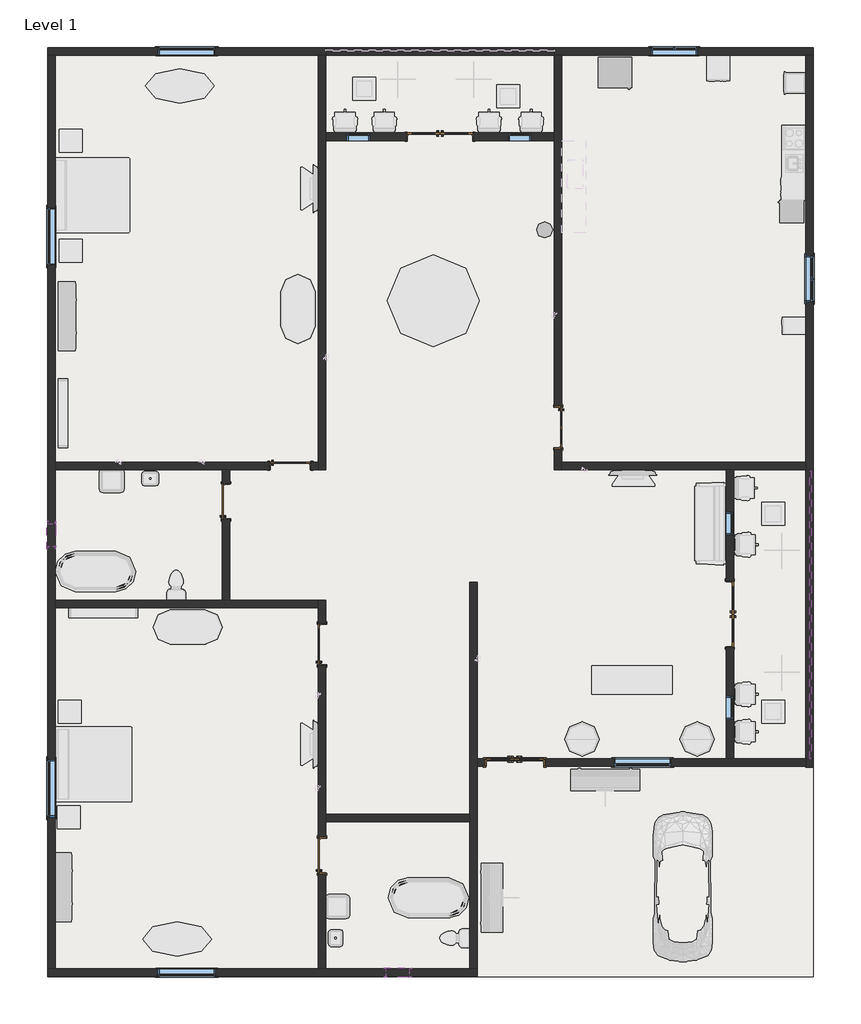
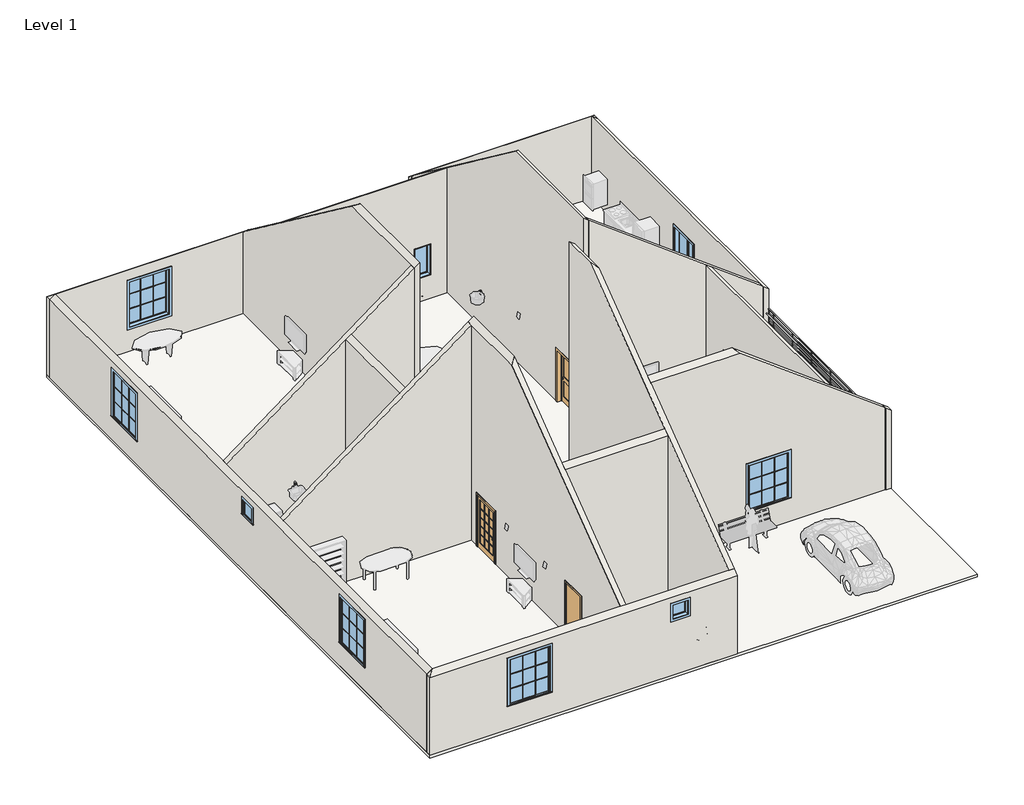
# One storey, part 1 of 2: 20 walls, 13 windows, 8 doors, 1 railing, 1 slab.
"""IFC4 building model written with IfcOpenShell, lengths in millimetres."""

from ifc_helpers import new_model, si_unit, point, frame, frame_2d, origin, origin_with_axes, place, context, project, spatial, polyline, circle_curve, trimmed, segment, composite_curve, outline, extrude, faceted_brep, transform, mapped, element, save
from components import door_b03bd389, door_146fce4d, door_63baf7d0, door_797b0c7a, door_f3911013, window_cc15f82e, window_0862ab64, window_9110666e, window_80bd9af0, window_e41d21a6

model = new_model("IFC4")

# Units and contexts
model_context = context("Model", 3, world=origin())
ifc_project = project(units=[si_unit("LENGTHUNIT", "METRE", prefix="MILLI")], contexts=[model_context])

# Site, building, storey
site = spatial("IfcSite", under=ifc_project)
building = spatial("IfcBuilding", under=site)
storey = spatial("IfcBuildingStorey", under=building, Name="Level 1", Elevation=0.0)

# Doors
placement = place(None, origin())
door_shape = door_b03bd389(model_context)
element("IfcDoor", 1, ObjectType="Door-Exterior-Double-Full Glass-Wood_Clad : 60\" x 80\"", at=placement, inside=storey, context=model_context, shape_type="MappedRepresentation", body=[
    mapped(door_shape, transform((-2295.8295712, -8019.3204109, 0.0), x_axis=(1.0, 0.0, 0.0), y_axis=(0.0, 1.0, 0.0), z_axis=(0.0, 0.0, 1.0))),
])
door_2_shape = door_146fce4d(model_context)
element("IfcDoor", 2, ObjectType="Door-Interior-Double-Full Glass-Wood : 68\" x 80\"", at=placement, inside=storey, context=model_context, shape_type="MappedRepresentation", body=[
    mapped(door_2_shape, transform((-4277.0295712, 8541.4795891, 0.0), x_axis=(1.0, 0.0, 0.0), y_axis=(0.0, 1.0, 0.0), z_axis=(0.0, 0.0, 1.0))),
])
element("IfcDoor", 3, ObjectType="Door-Interior-Double-Full Glass-Wood : 68\" x 80\"", at=placement, inside=storey, context=model_context, shape_type="MappedRepresentation", body=[
    mapped(door_2_shape, transform((3396.9454288, -4098.1954109, 0.0), x_axis=(0.0, -1.0, 0.0), y_axis=(1.0, 0.0, 0.0), z_axis=(0.0, 0.0, 1.0))),
])
door_3_shape = door_63baf7d0(model_context)
element("IfcDoor", 4, ObjectType="Door-Interior-Single-4_Panel-Wood : 42\" x 80\"", at=placement, inside=storey, context=model_context, shape_type="MappedRepresentation", body=[
    mapped(door_3_shape, transform((-1149.6545712, 842.1045891, 0.0), x_axis=(0.0, -1.0, 0.0), y_axis=(1.0, 0.0, 0.0), z_axis=(0.0, 0.0, 1.0))),
])
door_4_shape = door_797b0c7a(model_context)
element("IfcDoor", 5, ObjectType="Door-Interior-Single-Flush_Panel-Wood : 36\" x 80\"", at=placement, inside=storey, context=model_context, shape_type="MappedRepresentation", body=[
    mapped(door_4_shape, transform((-7404.4045712, -10486.2954109, 0.0), x_axis=(0.0, 1.0, 0.0), y_axis=(-1.0, 0.0, 0.0), z_axis=(0.0, 0.0, 1.0))),
])
element("IfcDoor", 6, ObjectType="Door-Interior-Single-Flush_Panel-Wood : 36\" x 80\"", at=placement, inside=storey, context=model_context, shape_type="MappedRepresentation", body=[
    mapped(door_4_shape, transform((-9944.4045712, -1113.6954109, 0.0), x_axis=(0.0, 1.0, 0.0), y_axis=(-1.0, 0.0, 0.0), z_axis=(0.0, 0.0, 1.0))),
])
door_5_shape = door_f3911013(model_context)
element("IfcDoor", 7, ObjectType="Door-Interior-Single-Full Glass-Wood : 42\" x 80\"", at=placement, inside=storey, context=model_context, shape_type="MappedRepresentation", body=[
    mapped(door_5_shape, transform((-8239.4295712, -170.7204109, 0.0), x_axis=(1.0, 0.0, 0.0), y_axis=(0.0, 1.0, 0.0), z_axis=(0.0, 0.0, 1.0))),
])
element("IfcDoor", 8, ObjectType="Door-Interior-Single-Full Glass-Wood : 42\" x 80\"", at=placement, inside=storey, context=model_context, shape_type="MappedRepresentation", body=[
    mapped(door_5_shape, transform((-7404.4045712, -4898.2954109, 0.0), x_axis=(0.0, 1.0, 0.0), y_axis=(-1.0, 0.0, 0.0), z_axis=(0.0, 0.0, 1.0))),
])

# Railing
element("IfcRailing", 9, ObjectType="Guardrail - Pipe", at=placement, inside=storey, context=model_context, shape_type="SweptSolid", body=[
    extrude(outline(composite_curve([segment(trimmed(circle_curve(frame_2d((2114.55, 5527.3704288)), 19.05), [point((2114.55, 5546.4204288))], [point((2114.55, 5508.3204288))], False, "CARTESIAN"), True, "CONTINUOUS"), segment(trimmed(circle_curve(frame_2d((2114.55, 5527.3704288)), 19.05), [point((2114.55, 5508.3204288))], [point((2114.55, 5546.4204288))], False, "CARTESIAN"), True, "CONTINUOUS")], self_intersect=False)), frame((0.0, -7920.8954109, 0.0), z_axis=(0.0, 1.0, 0.0), x_axis=(0.0, 0.0, 1.0)), (0.0, 0.0, 1.0), 7620.0),
    extrude(outline(composite_curve([segment(trimmed(circle_curve(frame_2d((2266.95, 5603.5704288)), 19.05), [point((2266.95, 5622.6204288))], [point((2266.95, 5584.5204288))], False, "CARTESIAN"), True, "CONTINUOUS"), segment(trimmed(circle_curve(frame_2d((2266.95, 5603.5704288)), 19.05), [point((2266.95, 5584.5204288))], [point((2266.95, 5622.6204288))], False, "CARTESIAN"), True, "CONTINUOUS")], self_intersect=False)), frame((0.0, -7920.8954109, 0.0), z_axis=(0.0, 1.0, 0.0), x_axis=(0.0, 0.0, 1.0)), (0.0, 0.0, 1.0), 7620.0),
    extrude(outline(composite_curve([segment(trimmed(circle_curve(frame_2d((2120.9, 5603.5704288)), 12.7), [point((2120.9, 5590.8704288))], [point((2120.9, 5616.2704288))], False, "CARTESIAN"), True, "CONTINUOUS"), segment(trimmed(circle_curve(frame_2d((2120.9, 5603.5704288)), 12.7), [point((2120.9, 5616.2704288))], [point((2120.9, 5590.8704288))], False, "CARTESIAN"), True, "CONTINUOUS")], self_intersect=False)), frame((0.0, -7920.8954109, 0.0), z_axis=(0.0, 1.0, 0.0), x_axis=(0.0, 0.0, 1.0)), (0.0, 0.0, 1.0), 7620.0),
    extrude(outline(composite_curve([segment(trimmed(circle_curve(frame_2d((1993.9, 5603.5704288)), 12.7), [point((1993.9, 5590.8704288))], [point((1993.9, 5616.2704288))], False, "CARTESIAN"), True, "CONTINUOUS"), segment(trimmed(circle_curve(frame_2d((1993.9, 5603.5704288)), 12.7), [point((1993.9, 5616.2704288))], [point((1993.9, 5590.8704288))], False, "CARTESIAN"), True, "CONTINUOUS")], self_intersect=False)), frame((0.0, -7920.8954109, 0.0), z_axis=(0.0, 1.0, 0.0), x_axis=(0.0, 0.0, 1.0)), (0.0, 0.0, 1.0), 7620.0),
    extrude(outline(composite_curve([segment(trimmed(circle_curve(frame_2d((1866.9, 5603.5704288)), 12.7), [point((1866.9, 5590.8704288))], [point((1866.9, 5616.2704288))], False, "CARTESIAN"), True, "CONTINUOUS"), segment(trimmed(circle_curve(frame_2d((1866.9, 5603.5704288)), 12.7), [point((1866.9, 5616.2704288))], [point((1866.9, 5590.8704288))], False, "CARTESIAN"), True, "CONTINUOUS")], self_intersect=False)), frame((0.0, -7920.8954109, 0.0), z_axis=(0.0, 1.0, 0.0), x_axis=(0.0, 0.0, 1.0)), (0.0, 0.0, 1.0), 7620.0),
    extrude(outline(composite_curve([segment(trimmed(circle_curve(frame_2d((1739.9, 5603.5704288)), 12.7), [point((1739.9, 5590.8704288))], [point((1739.9, 5616.2704288))], False, "CARTESIAN"), True, "CONTINUOUS"), segment(trimmed(circle_curve(frame_2d((1739.9, 5603.5704288)), 12.7), [point((1739.9, 5616.2704288))], [point((1739.9, 5590.8704288))], False, "CARTESIAN"), True, "CONTINUOUS")], self_intersect=False)), frame((0.0, -7920.8954109, 0.0), z_axis=(0.0, 1.0, 0.0), x_axis=(0.0, 0.0, 1.0)), (0.0, 0.0, 1.0), 7620.0),
    extrude(outline(composite_curve([segment(trimmed(circle_curve(frame_2d((1612.9, 5603.5704288)), 12.7), [point((1612.9, 5590.8704288))], [point((1612.9, 5616.2704288))], False, "CARTESIAN"), True, "CONTINUOUS"), segment(trimmed(circle_curve(frame_2d((1612.9, 5603.5704288)), 12.7), [point((1612.9, 5616.2704288))], [point((1612.9, 5590.8704288))], False, "CARTESIAN"), True, "CONTINUOUS")], self_intersect=False)), frame((0.0, -7920.8954109, 0.0), z_axis=(0.0, 1.0, 0.0), x_axis=(0.0, 0.0, 1.0)), (0.0, 0.0, 1.0), 7620.0),
    extrude(outline(composite_curve([segment(trimmed(circle_curve(frame_2d((1485.9, 5603.5704288)), 12.7), [point((1485.9, 5590.8704288))], [point((1485.9, 5616.2704288))], False, "CARTESIAN"), True, "CONTINUOUS"), segment(trimmed(circle_curve(frame_2d((1485.9, 5603.5704288)), 12.7), [point((1485.9, 5616.2704288))], [point((1485.9, 5590.8704288))], False, "CARTESIAN"), True, "CONTINUOUS")], self_intersect=False)), frame((0.0, -7920.8954109, 0.0), z_axis=(0.0, 1.0, 0.0), x_axis=(0.0, 0.0, 1.0)), (0.0, 0.0, 1.0), 7620.0),
    extrude(outline(composite_curve([segment(trimmed(circle_curve(frame_2d((1358.9, 5603.5704288)), 12.7), [point((1358.9, 5590.8704288))], [point((1358.9, 5616.2704288))], False, "CARTESIAN"), True, "CONTINUOUS"), segment(trimmed(circle_curve(frame_2d((1358.9, 5603.5704288)), 12.7), [point((1358.9, 5616.2704288))], [point((1358.9, 5590.8704288))], False, "CARTESIAN"), True, "CONTINUOUS")], self_intersect=False)), frame((0.0, -7920.8954109, 0.0), z_axis=(0.0, 1.0, 0.0), x_axis=(0.0, 0.0, 1.0)), (0.0, 0.0, 1.0), 7620.0),
    extrude(outline(composite_curve([segment(trimmed(circle_curve(frame_2d((5603.5704288, -605.6954109)), 12.7), [point((5590.8704288, -605.6954109))], [point((5616.2704288, -605.6954109))], False, "CARTESIAN"), True, "CONTINUOUS"), segment(trimmed(circle_curve(frame_2d((5603.5704288, -605.6954109)), 12.7), [point((5616.2704288, -605.6954109))], [point((5590.8704288, -605.6954109))], False, "CARTESIAN"), True, "CONTINUOUS")], self_intersect=False)), frame((0.0, 0.0, 1219.2), z_axis=(0.0, 0.0, 1.0), x_axis=(1.0, 0.0, 0.0)), (0.0, 0.0, 1.0), 1028.7),
    extrude(outline(composite_curve([segment(trimmed(circle_curve(frame_2d((5603.5704288, -1824.8954109)), 12.7), [point((5590.8704288, -1824.8954109))], [point((5616.2704288, -1824.8954109))], False, "CARTESIAN"), True, "CONTINUOUS"), segment(trimmed(circle_curve(frame_2d((5603.5704288, -1824.8954109)), 12.7), [point((5616.2704288, -1824.8954109))], [point((5590.8704288, -1824.8954109))], False, "CARTESIAN"), True, "CONTINUOUS")], self_intersect=False)), frame((0.0, 0.0, 1219.2), z_axis=(0.0, 0.0, 1.0), x_axis=(1.0, 0.0, 0.0)), (0.0, 0.0, 1.0), 1028.7),
    extrude(outline(composite_curve([segment(trimmed(circle_curve(frame_2d((5603.5704288, -3044.0954109)), 12.7), [point((5590.8704288, -3044.0954109))], [point((5616.2704288, -3044.0954109))], False, "CARTESIAN"), True, "CONTINUOUS"), segment(trimmed(circle_curve(frame_2d((5603.5704288, -3044.0954109)), 12.7), [point((5616.2704288, -3044.0954109))], [point((5590.8704288, -3044.0954109))], False, "CARTESIAN"), True, "CONTINUOUS")], self_intersect=False)), frame((0.0, 0.0, 1219.2), z_axis=(0.0, 0.0, 1.0), x_axis=(1.0, 0.0, 0.0)), (0.0, 0.0, 1.0), 1028.7),
    extrude(outline(composite_curve([segment(trimmed(circle_curve(frame_2d((5603.5704288, -4263.2954109)), 12.7), [point((5590.8704288, -4263.2954109))], [point((5616.2704288, -4263.2954109))], False, "CARTESIAN"), True, "CONTINUOUS"), segment(trimmed(circle_curve(frame_2d((5603.5704288, -4263.2954109)), 12.7), [point((5616.2704288, -4263.2954109))], [point((5590.8704288, -4263.2954109))], False, "CARTESIAN"), True, "CONTINUOUS")], self_intersect=False)), frame((0.0, 0.0, 1219.2), z_axis=(0.0, 0.0, 1.0), x_axis=(1.0, 0.0, 0.0)), (0.0, 0.0, 1.0), 1028.7),
    extrude(outline(composite_curve([segment(trimmed(circle_curve(frame_2d((5603.5704288, -5482.4954109)), 12.7), [point((5590.8704288, -5482.4954109))], [point((5616.2704288, -5482.4954109))], False, "CARTESIAN"), True, "CONTINUOUS"), segment(trimmed(circle_curve(frame_2d((5603.5704288, -5482.4954109)), 12.7), [point((5616.2704288, -5482.4954109))], [point((5590.8704288, -5482.4954109))], False, "CARTESIAN"), True, "CONTINUOUS")], self_intersect=False)), frame((0.0, 0.0, 1219.2), z_axis=(0.0, 0.0, 1.0), x_axis=(1.0, 0.0, 0.0)), (0.0, 0.0, 1.0), 1028.7),
    extrude(outline(composite_curve([segment(trimmed(circle_curve(frame_2d((5603.5704288, -6701.6954109)), 12.7), [point((5590.8704288, -6701.6954109))], [point((5616.2704288, -6701.6954109))], False, "CARTESIAN"), True, "CONTINUOUS"), segment(trimmed(circle_curve(frame_2d((5603.5704288, -6701.6954109)), 12.7), [point((5616.2704288, -6701.6954109))], [point((5590.8704288, -6701.6954109))], False, "CARTESIAN"), True, "CONTINUOUS")], self_intersect=False)), frame((0.0, 0.0, 1219.2), z_axis=(0.0, 0.0, 1.0), x_axis=(1.0, 0.0, 0.0)), (0.0, 0.0, 1.0), 1028.7),
    extrude(outline(composite_curve([segment(trimmed(circle_curve(frame_2d((5603.5704288, -313.5954109)), 12.7), [point((5590.8704288, -313.5954109))], [point((5616.2704288, -313.5954109))], False, "CARTESIAN"), True, "CONTINUOUS"), segment(trimmed(circle_curve(frame_2d((5603.5704288, -313.5954109)), 12.7), [point((5616.2704288, -313.5954109))], [point((5590.8704288, -313.5954109))], False, "CARTESIAN"), True, "CONTINUOUS")], self_intersect=False)), frame((0.0, 0.0, 1219.2), z_axis=(0.0, 0.0, 1.0), x_axis=(1.0, 0.0, 0.0)), (0.0, 0.0, 1.0), 1028.7),
    extrude(outline(composite_curve([segment(trimmed(circle_curve(frame_2d((5603.5704288, -7908.1954109)), 12.7), [point((5590.8704288, -7908.1954109))], [point((5616.2704288, -7908.1954109))], False, "CARTESIAN"), True, "CONTINUOUS"), segment(trimmed(circle_curve(frame_2d((5603.5704288, -7908.1954109)), 12.7), [point((5616.2704288, -7908.1954109))], [point((5590.8704288, -7908.1954109))], False, "CARTESIAN"), True, "CONTINUOUS")], self_intersect=False)), frame((0.0, 0.0, 1219.2), z_axis=(0.0, 0.0, 1.0), x_axis=(1.0, 0.0, 0.0)), (0.0, 0.0, 1.0), 1028.7),
])

# Slab
element("IfcSlab", 10, ObjectType="LW Concrete on Metal Deck", at=placement, inside=storey, context=model_context, shape_type="SweptSolid", body=[
    extrude(outline(polyline([(5603.5704288, 10900.5045891), (5603.5704288, -13686.6954109), (-14665.6295712, -13686.6954109), (-14665.6295712, 10900.5045891), (5603.5704288, 10900.5045891)])), frame((0.0, 0.0, -104.775), z_axis=(0.0, 0.0, 1.0), x_axis=(1.0, 0.0, 0.0)), (0.0, 0.0, 1.0), 104.775),
])

# Walls
element("IfcWall", 11, ObjectType="Generic - 8\"", at=placement, inside=storey, context=model_context, shape_type="Brep", body=[
    faceted_brep([(-14665.6295712, 10697.3045891, 0.0), (-14462.4295712, 10697.3045891, 0.0), (-7502.8295712, 10697.3045891, 0.0), (-7299.6295712, 10697.3045891, 0.0), (-7299.6295712, 10697.3045891, 1219.2), (-7299.6295712, 10697.3045891, 3200.4), (-7502.8295712, 10697.3045891, 3200.4), (-14462.4295712, 10697.3045891, 3200.4), (-14665.6295712, 10697.3045891, 3048.0), (-10220.6295712, 10697.3045891, 2743.2), (-10220.6295712, 10697.3045891, 914.4), (-11744.6295712, 10697.3045891, 914.4), (-11744.6295712, 10697.3045891, 2743.2), (-14665.6295712, 10900.5045891, 0.0), (-14665.6295712, 10900.5045891, 3048.0), (-7299.6295712, 10900.5045891, 3048.0), (-7299.6295712, 10900.5045891, 1219.2), (-7299.6295712, 10900.5045891, 0.0), (-10220.6295712, 10900.5045891, 2743.2), (-11744.6295712, 10900.5045891, 2743.2), (-11744.6295712, 10900.5045891, 914.4), (-10220.6295712, 10900.5045891, 914.4)], [[[0, 1, 2, 3, 4, 5, 6, 7, 8], [9, 10, 11, 12]], [[13, 14, 15, 16, 17], [18, 19, 20, 21]], [[3, 2, 1, 0, 13, 17]], [[5, 4, 3, 17, 16, 15]], [[0, 8, 14, 13]], [[8, 7, 14]], [[7, 6, 5, 15, 14]], [[10, 9, 18, 21]], [[11, 10, 21, 20]], [[12, 11, 20, 19]], [[9, 12, 19, 18]]]),
])
element("IfcWall", 12, ObjectType="Generic - 8\"", at=placement, inside=storey, context=model_context, shape_type="Brep", body=[
    faceted_brep([(5400.3704288, 10697.3045891, 0.0), (5400.3704288, -72.2954109, 0.0), (5400.3704288, -275.4954109, 0.0), (5400.3704288, -300.8954109, 0.0), (5400.3704288, -300.8954109, 1219.2), (5400.3704288, -300.8954109, 3200.4), (5400.3704288, -275.4954109, 3200.4), (5400.3704288, -72.2954109, 3200.4), (5400.3704288, 10697.3045891, 3200.4), (5400.3704288, 4169.5045891, 2133.6), (5400.3704288, 4169.5045891, 914.4), (5400.3704288, 5388.7045891, 914.4), (5400.3704288, 5388.7045891, 2133.6), (5603.5704288, 10697.3045891, 0.0), (5603.5704288, 10697.3045891, 3048.0), (5603.5704288, -300.8954109, 3048.0), (5603.5704288, -300.8954109, 1219.2), (5603.5704288, -300.8954109, 0.0), (5603.5704288, 4169.5045891, 2133.6), (5603.5704288, 5388.7045891, 2133.6), (5603.5704288, 5388.7045891, 914.4), (5603.5704288, 4169.5045891, 914.4)], [[[0, 1, 2, 3, 4, 5, 6, 7, 8], [9, 10, 11, 12]], [[13, 14, 15, 16, 17], [18, 19, 20, 21]], [[3, 2, 1, 0, 13, 17]], [[5, 4, 3, 17, 16, 15]], [[0, 8, 14, 13]], [[8, 7, 6, 5, 15, 14]], [[10, 9, 18, 21]], [[11, 10, 21, 20]], [[12, 11, 20, 19]], [[9, 12, 19, 18]]]),
])
element("IfcWall", 13, ObjectType="Generic - 8\"", at=placement, inside=storey, context=model_context, shape_type="Brep", body=[
    faceted_brep([(-14462.4295712, -13483.4954109, 0.0), (-14462.4295712, -3933.0954109, 0.0), (-14462.4295712, -3729.8954109, 0.0), (-14462.4295712, -275.4954109, 0.0), (-14462.4295712, -72.2954109, 0.0), (-14462.4295712, 10697.3045891, 0.0), (-14462.4295712, 10697.3045891, 3200.4), (-14462.4295712, -72.2954109, 3200.4), (-14462.4295712, -275.4954109, 3200.4), (-14462.4295712, -3729.8954109, 3200.4), (-14462.4295712, -3933.0954109, 3200.4), (-14462.4295712, -13483.4954109, 3200.4), (-14462.4295712, -7946.2954109, 2743.2), (-14462.4295712, -7946.2954109, 914.4), (-14462.4295712, -9470.2954109, 914.4), (-14462.4295712, -9470.2954109, 2743.2), (-14462.4295712, 6658.7045891, 2743.2), (-14462.4295712, 6658.7045891, 914.4), (-14462.4295712, 5134.7045891, 914.4), (-14462.4295712, 5134.7045891, 2743.2), (-14462.4295712, -1697.8954109, 2768.6), (-14462.4295712, -1697.8954109, 2159.0), (-14462.4295712, -2307.4954109, 2159.0), (-14462.4295712, -2307.4954109, 2768.6), (-14665.6295712, -13483.4954109, 0.0), (-14665.6295712, -13483.4954109, 3048.0), (-14665.6295712, 10697.3045891, 3048.0), (-14665.6295712, 10697.3045891, 0.0), (-14665.6295712, -7946.2954109, 2743.2), (-14665.6295712, -9470.2954109, 2743.2), (-14665.6295712, -9470.2954109, 914.4), (-14665.6295712, -7946.2954109, 914.4), (-14665.6295712, 6658.7045891, 2743.2), (-14665.6295712, 5134.7045891, 2743.2), (-14665.6295712, 5134.7045891, 914.4), (-14665.6295712, 6658.7045891, 914.4), (-14665.6295712, -1697.8954109, 2768.6), (-14665.6295712, -2307.4954109, 2768.6), (-14665.6295712, -2307.4954109, 2159.0), (-14665.6295712, -1697.8954109, 2159.0)], [[[0, 1, 2, 3, 4, 5, 6, 7, 8, 9, 10, 11], [12, 13, 14, 15], [16, 17, 18, 19], [20, 21, 22, 23]], [[24, 25, 26, 27], [28, 29, 30, 31], [32, 33, 34, 35], [36, 37, 38, 39]], [[5, 4, 3, 2, 1, 0, 24, 27]], [[6, 5, 27, 26]], [[0, 11, 25, 24]], [[11, 10, 9, 8, 7, 6, 26, 25]], [[13, 12, 28, 31]], [[14, 13, 31, 30]], [[15, 14, 30, 29]], [[12, 15, 29, 28]], [[17, 16, 32, 35]], [[18, 17, 35, 34]], [[19, 18, 34, 33]], [[16, 19, 33, 32]], [[21, 20, 36, 39]], [[22, 21, 39, 38]], [[23, 22, 38, 37]], [[20, 23, 37, 36]]]),
])
element("IfcWall", 14, ObjectType="Generic - 8\"", at=placement, inside=storey, context=model_context, shape_type="Brep", body=[
    faceted_brep([(-7502.8295712, 10697.3045891, 3200.4), (-7502.8295712, 10697.3045891, 0.0), (-7502.8295712, -72.2954109, 0.0), (-7502.8295712, -275.4954109, 0.0), (-7502.8295712, -275.4954109, 8420.1), (-7502.8295712, -72.2954109, 8420.1), (-7502.8295712, 3737.7045891, 8420.1), (-7299.6295712, 10697.3045891, 0.0), (-7299.6295712, 10697.3045891, 3200.4), (-7299.6295712, 8639.9045891, 4743.45), (-7299.6295712, 8436.7045891, 4895.85), (-7299.6295712, 3534.5045891, 8572.5), (-7299.6295712, -275.4954109, 8572.5), (-7299.6295712, -275.4954109, 0.0), (-7299.6295712, 8436.7045891, 0.0), (-7299.6295712, 8639.9045891, 0.0)], [[[0, 1, 2, 3, 4, 5, 6]], [[7, 8, 9, 10, 11, 12, 13, 14, 15]], [[3, 2, 1, 7, 15, 14, 13]], [[4, 3, 13, 12]], [[0, 8, 7, 1]], [[0, 6, 11, 10, 9, 8]], [[6, 5, 4, 12, 11]]]),
])
element("IfcWall", 15, ObjectType="Generic - 8\"", at=placement, inside=storey, context=model_context, shape_type="Brep", body=[
    faceted_brep([(-1254.4295712, -275.4954109, 0.0), (-1254.4295712, -275.4954109, 8191.5), (-1254.4295712, 4042.5045891, 8191.5), (-1254.4295712, 8436.7045891, 4895.85), (-1254.4295712, 8639.9045891, 4743.45), (-1254.4295712, 10697.3045891, 3200.4), (-1254.4295712, 10697.3045891, 0.0), (-1254.4295712, 8639.9045891, 0.0), (-1254.4295712, 8436.7045891, 0.0), (-1254.4295712, 1400.9045891, 0.0), (-1254.4295712, 1400.9045891, 2057.4), (-1254.4295712, 283.3045891, 2057.4), (-1254.4295712, 283.3045891, 0.0), (-1051.2295712, -275.4954109, 8039.1), (-1051.2295712, -275.4954109, 0.0), (-1051.2295712, -72.2954109, 0.0), (-1051.2295712, 283.3045891, 0.0), (-1051.2295712, 283.3045891, 2057.4), (-1051.2295712, 1400.9045891, 2057.4), (-1051.2295712, 1400.9045891, 0.0), (-1051.2295712, 10697.3045891, 0.0), (-1051.2295712, 10697.3045891, 3200.4), (-1051.2295712, 4245.7045891, 8039.1), (-1051.2295712, -72.2954109, 8039.1)], [[[0, 1, 2, 3, 4, 5, 6, 7, 8, 9, 10, 11, 12]], [[13, 14, 15, 16, 17, 18, 19, 20, 21, 22, 23]], [[14, 0, 12, 16, 15]], [[6, 20, 19, 9, 8, 7]], [[1, 0, 14, 13]], [[5, 21, 20, 6]], [[21, 5, 4, 3, 2, 22]], [[1, 13, 23, 22, 2]], [[11, 17, 16, 12]], [[17, 11, 10, 18]], [[18, 10, 9, 19]]]),
])
element("IfcWall", 16, ObjectType="Generic - 8\"", at=placement, inside=storey, context=model_context, shape_type="Brep", body=[
    faceted_brep([(-14462.4295712, -275.4954109, 3200.4), (-14462.4295712, -275.4954109, 0.0), (-10042.8295712, -275.4954109, 0.0), (-9839.6295712, -275.4954109, 0.0), (-8798.2295712, -275.4954109, 0.0), (-8798.2295712, -275.4954109, 2057.4), (-7680.6295712, -275.4954109, 2057.4), (-7680.6295712, -275.4954109, 0.0), (-7502.8295712, -275.4954109, 0.0), (-7502.8295712, -275.4954109, 8420.1), (-9839.6295712, -275.4954109, 6667.5), (-10042.8295712, -275.4954109, 6515.1), (-14462.4295712, -72.2954109, 0.0), (-14462.4295712, -72.2954109, 3200.4), (-7502.8295712, -72.2954109, 8420.1), (-7502.8295712, -72.2954109, 0.0), (-7680.6295712, -72.2954109, 0.0), (-7680.6295712, -72.2954109, 2057.4), (-8798.2295712, -72.2954109, 2057.4), (-8798.2295712, -72.2954109, 0.0)], [[[0, 1, 2, 3, 4, 5, 6, 7, 8, 9, 10, 11]], [[12, 13, 14, 15, 16, 17, 18, 19]], [[1, 12, 19, 4, 3, 2]], [[15, 8, 7, 16]], [[1, 0, 13, 12]], [[9, 8, 15, 14]], [[0, 11, 10, 9, 14, 13]], [[6, 17, 16, 7]], [[17, 6, 5, 18]], [[18, 5, 4, 19]]]),
])
element("IfcWall", 17, ObjectType="Generic - 8\"", at=placement, inside=storey, context=model_context, shape_type="Brep", body=[
    faceted_brep([(-7502.8295712, -3729.8954109, 0.0), (-9839.6295712, -3729.8954109, 0.0), (-10042.8295712, -3729.8954109, 0.0), (-14462.4295712, -3729.8954109, 0.0), (-14462.4295712, -3729.8954109, 3200.4), (-10042.8295712, -3729.8954109, 6515.1), (-9839.6295712, -3729.8954109, 6667.5), (-7502.8295712, -3729.8954109, 8420.1), (-7502.8295712, -3933.0954109, 0.0), (-7502.8295712, -3933.0954109, 8420.1), (-14462.4295712, -3933.0954109, 3200.4), (-14462.4295712, -3933.0954109, 0.0)], [[[0, 1, 2, 3, 4, 5, 6, 7]], [[8, 9, 10, 11]], [[3, 2, 1, 0, 8, 11]], [[4, 3, 11, 10]], [[0, 7, 9, 8]], [[7, 6, 5, 4, 10, 9]]]),
])
element("IfcWall", 18, ObjectType="Generic - 8\"", at=placement, inside=storey, context=model_context, shape_type="Brep", body=[
    faceted_brep([(-7299.6295712, 8436.7045891, 4895.85), (-7299.6295712, 8436.7045891, 0.0), (-5166.0295712, 8436.7045891, 0.0), (-5166.0295712, 8436.7045891, 2057.4), (-3388.0295712, 8436.7045891, 2057.4), (-3388.0295712, 8436.7045891, 0.0), (-1254.4295712, 8436.7045891, 0.0), (-1254.4295712, 8436.7045891, 4895.85), (-6740.8295712, 8436.7045891, 2133.6), (-6131.2295712, 8436.7045891, 2133.6), (-6131.2295712, 8436.7045891, 914.4), (-6740.8295712, 8436.7045891, 914.4), (-1864.0295712, 8436.7045891, 2133.6), (-1864.0295712, 8436.7045891, 914.4), (-2473.6295712, 8436.7045891, 914.4), (-2473.6295712, 8436.7045891, 2133.6), (-7299.6295712, 8639.9045891, 0.0), (-7299.6295712, 8639.9045891, 4743.45), (-1254.4295712, 8639.9045891, 4743.45), (-1254.4295712, 8639.9045891, 0.0), (-3388.0295712, 8639.9045891, 0.0), (-3388.0295712, 8639.9045891, 2057.4), (-5166.0295712, 8639.9045891, 2057.4), (-5166.0295712, 8639.9045891, 0.0), (-6740.8295712, 8639.9045891, 2133.6), (-6740.8295712, 8639.9045891, 914.4), (-6131.2295712, 8639.9045891, 914.4), (-6131.2295712, 8639.9045891, 2133.6), (-1864.0295712, 8639.9045891, 2133.6), (-2473.6295712, 8639.9045891, 2133.6), (-2473.6295712, 8639.9045891, 914.4), (-1864.0295712, 8639.9045891, 914.4)], [[[0, 1, 2, 3, 4, 5, 6, 7], [8, 9, 10, 11], [12, 13, 14, 15]], [[16, 17, 18, 19, 20, 21, 22, 23], [24, 25, 26, 27], [28, 29, 30, 31]], [[1, 16, 23, 2]], [[19, 6, 5, 20]], [[1, 0, 17, 16]], [[7, 6, 19, 18]], [[0, 7, 18, 17]], [[4, 21, 20, 5]], [[21, 4, 3, 22]], [[22, 3, 2, 23]], [[25, 24, 8, 11]], [[26, 25, 11, 10]], [[27, 26, 10, 9]], [[24, 27, 9, 8]], [[13, 12, 28, 31]], [[14, 13, 31, 30]], [[15, 14, 30, 29]], [[12, 15, 29, 28]]]),
])
element("IfcWall", 19, ObjectType="Generic - 8\"", at=placement, inside=storey, context=model_context, shape_type="Brep", body=[
    faceted_brep([(-1051.2295712, -275.4954109, 0.0), (3292.1704288, -275.4954109, 0.0), (3495.3704288, -275.4954109, 0.0), (5400.3704288, -275.4954109, 0.0), (5400.3704288, -275.4954109, 3200.4), (3495.3704288, -275.4954109, 4629.15), (3292.1704288, -275.4954109, 4781.55), (-1051.2295712, -275.4954109, 8039.1), (-1051.2295712, -72.2954109, 0.0), (-1051.2295712, -72.2954109, 8039.1), (5400.3704288, -72.2954109, 3200.4), (5400.3704288, -72.2954109, 0.0)], [[[0, 1, 2, 3, 4, 5, 6, 7]], [[8, 9, 10, 11]], [[3, 2, 1, 0, 8, 11]], [[4, 3, 11, 10]], [[0, 7, 9, 8]], [[7, 6, 5, 4, 10, 9]]]),
])
element("IfcWall", 20, ObjectType="Generic - 8\"", at=placement, inside=storey, context=model_context, shape_type="Brep", body=[
    faceted_brep([(-3286.4295712, -7920.8954109, 0.0), (-3286.4295712, -7920.8954109, 7372.35), (-162.2295712, -7920.8954109, 7372.35), (3292.1704288, -7920.8954109, 4781.55), (3495.3704288, -7920.8954109, 4629.15), (5400.3704288, -7920.8954109, 3200.4), (5400.3704288, -7920.8954109, 0.0), (3495.3704288, -7920.8954109, 0.0), (3292.1704288, -7920.8954109, 0.0), (-1508.4295712, -7920.8954109, 0.0), (-1508.4295712, -7920.8954109, 2057.4), (-3083.2295712, -7920.8954109, 2057.4), (-3083.2295712, -7920.8954109, 0.0), (320.3704288, -7920.8954109, 2743.2), (320.3704288, -7920.8954109, 914.4), (1844.3704288, -7920.8954109, 914.4), (1844.3704288, -7920.8954109, 2743.2), (-3286.4295712, -8124.0954109, 7219.95), (-3286.4295712, -8124.0954109, 0.0), (-3083.2295712, -8124.0954109, 0.0), (-3083.2295712, -8124.0954109, 2057.4), (-1508.4295712, -8124.0954109, 2057.4), (-1508.4295712, -8124.0954109, 0.0), (5400.3704288, -8124.0954109, 0.0), (5400.3704288, -8124.0954109, 3200.4), (40.9704288, -8124.0954109, 7219.95), (320.3704288, -8124.0954109, 2743.2), (1844.3704288, -8124.0954109, 2743.2), (1844.3704288, -8124.0954109, 914.4), (320.3704288, -8124.0954109, 914.4)], [[[0, 1, 2, 3, 4, 5, 6, 7, 8, 9, 10, 11, 12], [13, 14, 15, 16]], [[17, 18, 19, 20, 21, 22, 23, 24, 25], [26, 27, 28, 29]], [[6, 23, 22, 9, 8, 7]], [[18, 0, 12, 19]], [[1, 0, 18, 17]], [[5, 24, 23, 6]], [[24, 5, 4, 3, 2, 25]], [[1, 17, 25, 2]], [[21, 10, 9, 22]], [[10, 21, 20, 11]], [[11, 20, 19, 12]], [[14, 13, 26, 29]], [[15, 14, 29, 28]], [[16, 15, 28, 27]], [[13, 16, 27, 26]]]),
])
element("IfcWall", 21, ObjectType="Generic - 8\"", at=placement, inside=storey, context=model_context, shape_type="Brep", body=[
    faceted_brep([(3292.1704288, -275.4954109, 4781.55), (3292.1704288, -275.4954109, 0.0), (3292.1704288, -3209.1954109, 0.0), (3292.1704288, -3209.1954109, 2057.4), (3292.1704288, -4987.1954109, 2057.4), (3292.1704288, -4987.1954109, 0.0), (3292.1704288, -7920.8954109, 0.0), (3292.1704288, -7920.8954109, 4781.55), (3292.1704288, -2002.6954109, 2133.6), (3292.1704288, -2002.6954109, 914.4), (3292.1704288, -1393.0954109, 914.4), (3292.1704288, -1393.0954109, 2133.6), (3292.1704288, -6879.4954109, 2133.6), (3292.1704288, -6879.4954109, 914.4), (3292.1704288, -6269.8954109, 914.4), (3292.1704288, -6269.8954109, 2133.6), (3495.3704288, -275.4954109, 0.0), (3495.3704288, -275.4954109, 4629.15), (3495.3704288, -7920.8954109, 4629.15), (3495.3704288, -7920.8954109, 0.0), (3495.3704288, -4987.1954109, 0.0), (3495.3704288, -4987.1954109, 2057.4), (3495.3704288, -3209.1954109, 2057.4), (3495.3704288, -3209.1954109, 0.0), (3495.3704288, -2002.6954109, 2133.6), (3495.3704288, -1393.0954109, 2133.6), (3495.3704288, -1393.0954109, 914.4), (3495.3704288, -2002.6954109, 914.4), (3495.3704288, -6879.4954109, 2133.6), (3495.3704288, -6269.8954109, 2133.6), (3495.3704288, -6269.8954109, 914.4), (3495.3704288, -6879.4954109, 914.4)], [[[0, 1, 2, 3, 4, 5, 6, 7], [8, 9, 10, 11], [12, 13, 14, 15]], [[16, 17, 18, 19, 20, 21, 22, 23], [24, 25, 26, 27], [28, 29, 30, 31]], [[1, 16, 23, 2]], [[19, 6, 5, 20]], [[1, 0, 17, 16]], [[7, 6, 19, 18]], [[0, 7, 18, 17]], [[4, 21, 20, 5]], [[21, 4, 3, 22]], [[22, 3, 2, 23]], [[9, 8, 24, 27]], [[10, 9, 27, 26]], [[11, 10, 26, 25]], [[8, 11, 25, 24]], [[13, 12, 28, 31]], [[14, 13, 31, 30]], [[15, 14, 30, 29]], [[12, 15, 29, 28]]]),
])
element("IfcWall", 22, ObjectType="Generic - 8\"", at=placement, inside=storey, context=model_context, shape_type="Brep", body=[
    faceted_brep([(-3286.4295712, -13483.4954109, 0.0), (-3286.4295712, -8124.0954109, 0.0), (-3286.4295712, -7920.8954109, 0.0), (-3286.4295712, -3247.2954109, 0.0), (-3286.4295712, -3247.2954109, 9715.5), (-3286.4295712, -4796.6954109, 9715.5), (-3286.4295712, -7920.8954109, 7372.35), (-3286.4295712, -8124.0954109, 7219.95), (-3286.4295712, -13483.4954109, 3200.4), (-3489.6295712, -13483.4954109, 0.0), (-3489.6295712, -13483.4954109, 3200.4), (-3489.6295712, -9597.2954109, 6115.05), (-3489.6295712, -9394.0954109, 6267.45), (-3489.6295712, -4593.4954109, 9867.9), (-3489.6295712, -3247.2954109, 9867.9), (-3489.6295712, -3247.2954109, 0.0), (-3489.6295712, -9394.0954109, 0.0), (-3489.6295712, -9597.2954109, 0.0)], [[[0, 1, 2, 3, 4, 5, 6, 7, 8]], [[9, 10, 11, 12, 13, 14, 15, 16, 17]], [[3, 2, 1, 0, 9, 17, 16, 15]], [[4, 3, 15, 14]], [[0, 8, 10, 9]], [[8, 7, 6, 5, 13, 12, 11, 10]], [[5, 4, 14, 13]]]),
])
element("IfcWall", 23, ObjectType="Generic - 8\"", at=placement, inside=storey, context=model_context, shape_type="Brep", body=[
    faceted_brep([(-3286.4295712, -13483.4954109, 0.0), (-3489.6295712, -13483.4954109, 0.0), (-7299.6295712, -13483.4954109, 0.0), (-7502.8295712, -13483.4954109, 0.0), (-14462.4295712, -13483.4954109, 0.0), (-14665.6295712, -13483.4954109, 0.0), (-14665.6295712, -13483.4954109, 3048.0), (-14462.4295712, -13483.4954109, 3200.4), (-7502.8295712, -13483.4954109, 3200.4), (-7299.6295712, -13483.4954109, 3200.4), (-3489.6295712, -13483.4954109, 3200.4), (-3286.4295712, -13483.4954109, 3200.4), (-11744.6295712, -13483.4954109, 2743.2), (-11744.6295712, -13483.4954109, 914.4), (-10220.6295712, -13483.4954109, 914.4), (-10220.6295712, -13483.4954109, 2743.2), (-5089.8295712, -13483.4954109, 2768.6), (-5699.4295712, -13483.4954109, 2768.6), (-5699.4295712, -13483.4954109, 2159.0), (-5089.8295712, -13483.4954109, 2159.0), (-3286.4295712, -13686.6954109, 0.0), (-3286.4295712, -13686.6954109, 3048.0), (-14665.6295712, -13686.6954109, 3048.0), (-14665.6295712, -13686.6954109, 0.0), (-11744.6295712, -13686.6954109, 2743.2), (-10220.6295712, -13686.6954109, 2743.2), (-10220.6295712, -13686.6954109, 914.4), (-11744.6295712, -13686.6954109, 914.4), (-5089.8295712, -13686.6954109, 2768.6), (-5089.8295712, -13686.6954109, 2159.0), (-5699.4295712, -13686.6954109, 2159.0), (-5699.4295712, -13686.6954109, 2768.6)], [[[0, 1, 2, 3, 4, 5, 6, 7, 8, 9, 10, 11], [12, 13, 14, 15], [16, 17, 18, 19]], [[20, 21, 22, 23], [24, 25, 26, 27], [28, 29, 30, 31]], [[5, 4, 3, 2, 1, 0, 20, 23]], [[0, 11, 21, 20]], [[6, 5, 23, 22]], [[11, 10, 9, 8, 7, 22, 21]], [[7, 6, 22]], [[13, 12, 24, 27]], [[14, 13, 27, 26]], [[15, 14, 26, 25]], [[12, 15, 25, 24]], [[29, 28, 16, 19]], [[30, 29, 19, 18]], [[31, 30, 18, 17]], [[28, 31, 17, 16]]]),
])
element("IfcWall", 24, ObjectType="Generic - 8\"", at=placement, inside=storey, context=model_context, shape_type="SweptSolid", body=[
    extrude(outline(polyline([(-9394.0954109, 6267.45), (-9394.0954109, 0.0), (-9597.2954109, 0.0), (-9597.2954109, 6115.05), (-9394.0954109, 6267.45)])), frame((-7299.6295712, 0.0, 0.0), z_axis=(1.0, 0.0, 0.0), x_axis=(0.0, 1.0, 0.0)), (0.0, 0.0, 1.0), 3810.0),
])
element("IfcWall", 25, ObjectType="Generic - 8\"", at=placement, inside=storey, context=model_context, shape_type="Brep", body=[
    faceted_brep([(-7502.8295712, -3729.8954109, 8420.1), (-7502.8295712, -3729.8954109, 0.0), (-7502.8295712, -3933.0954109, 0.0), (-7502.8295712, -4339.4954109, 0.0), (-7502.8295712, -4339.4954109, 2057.4), (-7502.8295712, -5457.0954109, 2057.4), (-7502.8295712, -5457.0954109, 0.0), (-7502.8295712, -10003.6954109, 0.0), (-7502.8295712, -10003.6954109, 2057.4), (-7502.8295712, -10968.8954109, 2057.4), (-7502.8295712, -10968.8954109, 0.0), (-7502.8295712, -13483.4954109, 0.0), (-7502.8295712, -13483.4954109, 3200.4), (-7502.8295712, -6523.8954109, 8420.1), (-7502.8295712, -3933.0954109, 8420.1), (-7299.6295712, -3729.8954109, 0.0), (-7299.6295712, -3729.8954109, 8572.5), (-7299.6295712, -6320.6954109, 8572.5), (-7299.6295712, -9394.0954109, 6267.45), (-7299.6295712, -9597.2954109, 6115.05), (-7299.6295712, -13483.4954109, 3200.4), (-7299.6295712, -13483.4954109, 0.0), (-7299.6295712, -10968.8954109, 0.0), (-7299.6295712, -10968.8954109, 2057.4), (-7299.6295712, -10003.6954109, 2057.4), (-7299.6295712, -10003.6954109, 0.0), (-7299.6295712, -9597.2954109, 0.0), (-7299.6295712, -9394.0954109, 0.0), (-7299.6295712, -5457.0954109, 0.0), (-7299.6295712, -5457.0954109, 2057.4), (-7299.6295712, -4339.4954109, 2057.4), (-7299.6295712, -4339.4954109, 0.0)], [[[0, 1, 2, 3, 4, 5, 6, 7, 8, 9, 10, 11, 12, 13, 14]], [[15, 16, 17, 18, 19, 20, 21, 22, 23, 24, 25, 26, 27, 28, 29, 30, 31]], [[1, 15, 31, 3, 2]], [[21, 11, 10, 22]], [[25, 7, 6, 28, 27, 26]], [[1, 0, 16, 15]], [[12, 11, 21, 20]], [[16, 0, 14, 13, 17]], [[12, 20, 19, 18, 17, 13]], [[24, 8, 7, 25]], [[8, 24, 23, 9]], [[9, 23, 22, 10]], [[30, 4, 3, 31]], [[4, 30, 29, 5]], [[5, 29, 28, 6]]]),
])
element("IfcWall", 26, ObjectType="Generic - 8\"", at=placement, inside=storey, context=model_context, shape_type="Brep", body=[
    faceted_brep([(-10042.8295712, -275.4954109, 6515.1), (-10042.8295712, -275.4954109, 0.0), (-10042.8295712, -631.0954109, 0.0), (-10042.8295712, -631.0954109, 2057.4), (-10042.8295712, -1596.2954109, 2057.4), (-10042.8295712, -1596.2954109, 0.0), (-10042.8295712, -3729.8954109, 0.0), (-10042.8295712, -3729.8954109, 6515.1), (-9839.6295712, -275.4954109, 0.0), (-9839.6295712, -275.4954109, 6667.5), (-9839.6295712, -3729.8954109, 6667.5), (-9839.6295712, -3729.8954109, 0.0), (-9839.6295712, -1596.2954109, 0.0), (-9839.6295712, -1596.2954109, 2057.4), (-9839.6295712, -631.0954109, 2057.4), (-9839.6295712, -631.0954109, 0.0)], [[[0, 1, 2, 3, 4, 5, 6, 7]], [[8, 9, 10, 11, 12, 13, 14, 15]], [[1, 8, 15, 2]], [[11, 6, 5, 12]], [[1, 0, 9, 8]], [[7, 6, 11, 10]], [[0, 7, 10, 9]], [[14, 3, 2, 15]], [[3, 14, 13, 4]], [[4, 13, 12, 5]]]),
])
element("IfcWall", 27, ObjectType="Generic - 8\"", at=placement, inside=storey, context=model_context, shape_type="SweptSolid", body=[
    extrude(outline(polyline([(-1254.4295712, 10697.3045891), (-7299.6295712, 10697.3045891), (-7299.6295712, 10900.5045891), (-1254.4295712, 10900.5045891), (-1254.4295712, 10697.3045891)])), origin_with_axes(), (0.0, 0.0, 1.0), 1219.2),
])
element("IfcWall", 28, ObjectType="Generic - 8\"", at=placement, inside=storey, context=model_context, shape_type="Brep", body=[
    faceted_brep([(-1254.4295712, 10697.3045891, 0.0), (-1051.2295712, 10697.3045891, 0.0), (5400.3704288, 10697.3045891, 0.0), (5603.5704288, 10697.3045891, 0.0), (5603.5704288, 10697.3045891, 3048.0), (5400.3704288, 10697.3045891, 3200.4), (-1051.2295712, 10697.3045891, 3200.4), (-1254.4295712, 10697.3045891, 3200.4), (-1254.4295712, 10697.3045891, 1219.2), (2530.1704288, 10697.3045891, 2133.6), (2530.1704288, 10697.3045891, 914.4), (1310.9704288, 10697.3045891, 914.4), (1310.9704288, 10697.3045891, 2133.6), (-1254.4295712, 10900.5045891, 0.0), (-1254.4295712, 10900.5045891, 1219.2), (-1254.4295712, 10900.5045891, 3048.0), (5603.5704288, 10900.5045891, 3048.0), (5603.5704288, 10900.5045891, 0.0), (2530.1704288, 10900.5045891, 2133.6), (1310.9704288, 10900.5045891, 2133.6), (1310.9704288, 10900.5045891, 914.4), (2530.1704288, 10900.5045891, 914.4)], [[[0, 1, 2, 3, 4, 5, 6, 7, 8], [9, 10, 11, 12]], [[13, 14, 15, 16, 17], [18, 19, 20, 21]], [[3, 2, 1, 0, 13, 17]], [[0, 8, 7, 15, 14, 13]], [[4, 3, 17, 16]], [[7, 6, 5, 16, 15]], [[5, 4, 16]], [[10, 9, 18, 21]], [[11, 10, 21, 20]], [[12, 11, 20, 19]], [[9, 12, 19, 18]]]),
])
element("IfcWall", 29, ObjectType="Generic - 8\"", at=placement, inside=storey, context=model_context, shape_type="SweptSolid", body=[
    extrude(outline(polyline([(5400.3704288, -7920.8954109), (5400.3704288, -300.8954109), (5603.5704288, -300.8954109), (5603.5704288, -7920.8954109), (5400.3704288, -7920.8954109)])), origin_with_axes(), (0.0, 0.0, 1.0), 1219.2),
])
element("IfcWall", 30, ObjectType="Generic - 8\"", at=placement, inside=storey, context=model_context, shape_type="Brep", body=[
    faceted_brep([(5400.3704288, -7920.8954109, 0.0), (5400.3704288, -8124.0954109, 0.0), (5400.3704288, -8149.4954109, 0.0), (5400.3704288, -8149.4954109, 3200.4), (5400.3704288, -8124.0954109, 3200.4), (5400.3704288, -7920.8954109, 3200.4), (5400.3704288, -7920.8954109, 1219.2), (5603.5704288, -7920.8954109, 0.0), (5603.5704288, -7920.8954109, 1219.2), (5603.5704288, -7920.8954109, 3048.0), (5603.5704288, -8149.4954109, 3048.0), (5603.5704288, -8149.4954109, 0.0)], [[[0, 1, 2, 3, 4, 5, 6]], [[7, 8, 9, 10, 11]], [[2, 1, 0, 7, 11]], [[3, 2, 11, 10]], [[0, 6, 5, 9, 8, 7]], [[5, 4, 3, 10, 9]]]),
])

# Windows
window_shape = window_cc15f82e(model_context)
element("IfcWindow", 31, ObjectType="Casement 3x3 with Trim : 60\" x 72\"", at=placement, inside=storey, context=model_context, shape_type="MappedRepresentation", body=[
    mapped(window_shape, transform((1082.3704288, -8022.4954109, 609.6), x_axis=(-1.0, 0.0, 0.0), y_axis=(0.0, -1.0, 0.0), z_axis=(0.0, 0.0, 1.0))),
])
element("IfcWindow", 32, ObjectType="Casement 3x3 with Trim : 60\" x 72\"", at=placement, inside=storey, context=model_context, shape_type="MappedRepresentation", body=[
    mapped(window_shape, transform((-10982.6295712, -13585.0954109, 609.6), x_axis=(-1.0, 0.0, 0.0), y_axis=(0.0, -1.0, 0.0), z_axis=(0.0, 0.0, 1.0))),
])
element("IfcWindow", 33, ObjectType="Casement 3x3 with Trim : 60\" x 72\"", at=placement, inside=storey, context=model_context, shape_type="MappedRepresentation", body=[
    mapped(window_shape, transform((-14564.0295712, -8708.2954109, 609.6), x_axis=(0.0, 1.0, 0.0), y_axis=(-1.0, 0.0, 0.0), z_axis=(0.0, 0.0, 1.0))),
])
element("IfcWindow", 34, ObjectType="Casement 3x3 with Trim : 60\" x 72\"", at=placement, inside=storey, context=model_context, shape_type="MappedRepresentation", body=[
    mapped(window_shape, transform((-14564.0295712, 5896.7045891, 609.6), x_axis=(0.0, 1.0, 0.0), y_axis=(-1.0, 0.0, 0.0), z_axis=(0.0, 0.0, 1.0))),
])
element("IfcWindow", 35, ObjectType="Casement 3x3 with Trim : 60\" x 72\"", at=placement, inside=storey, context=model_context, shape_type="MappedRepresentation", body=[
    mapped(window_shape, transform((-10982.6295712, 10798.9045891, 609.6), x_axis=(1.0, 0.0, 0.0), y_axis=(0.0, 1.0, 0.0), z_axis=(0.0, 0.0, 1.0))),
])
window_2_shape = window_0862ab64(model_context)
element("IfcWindow", 36, ObjectType="Casement Dbl with Trim : 48\" x 48\"", at=placement, inside=storey, context=model_context, shape_type="MappedRepresentation", body=[
    mapped(window_2_shape, transform((5482.9204288, 4779.1045891, 0.0), x_axis=(0.0, -1.0, 0.0), y_axis=(1.0, 0.0, 0.0), z_axis=(0.0, 0.0, 1.0))),
])
element("IfcWindow", 37, ObjectType="Casement Dbl with Trim : 48\" x 48\"", at=placement, inside=storey, context=model_context, shape_type="MappedRepresentation", body=[
    mapped(window_2_shape, transform((1920.5704288, 10779.8545891, 0.0), x_axis=(1.0, 0.0, 0.0), y_axis=(0.0, 1.0, 0.0), z_axis=(0.0, 0.0, 1.0))),
])
window_3_shape = window_9110666e(model_context)
element("IfcWindow", 38, ObjectType="Fixed : 24\" x 48\"", at=placement, inside=storey, context=model_context, shape_type="MappedRepresentation", body=[
    mapped(window_3_shape, transform((-6474.1295712, 8538.3045891, 0.0), x_axis=(-1.0, 0.0, 0.0), y_axis=(0.0, -1.0, 0.0), z_axis=(0.0, 0.0, 1.0))),
])
window_4_shape = window_80bd9af0(model_context)
element("IfcWindow", 39, ObjectType="Fixed : 24\" x 48\"", at=placement, inside=storey, context=model_context, shape_type="MappedRepresentation", body=[
    mapped(window_4_shape, transform((-2130.7295712, 8538.3045891, 0.0), x_axis=(1.0, 0.0, 0.0), y_axis=(0.0, 1.0, 0.0), z_axis=(0.0, 0.0, 1.0))),
])
element("IfcWindow", 40, ObjectType="Fixed : 24\" x 48\"", at=placement, inside=storey, context=model_context, shape_type="MappedRepresentation", body=[
    mapped(window_4_shape, transform((3393.7704288, -1735.9954109, 0.0), x_axis=(0.0, -1.0, 0.0), y_axis=(1.0, 0.0, 0.0), z_axis=(0.0, 0.0, 1.0))),
])
element("IfcWindow", 41, ObjectType="Fixed : 24\" x 48\"", at=placement, inside=storey, context=model_context, shape_type="MappedRepresentation", body=[
    mapped(window_4_shape, transform((3393.7704288, -6612.7954109, 0.0), x_axis=(0.0, -1.0, 0.0), y_axis=(1.0, 0.0, 0.0), z_axis=(0.0, 0.0, 1.0))),
])
window_5_shape = window_e41d21a6(model_context)
element("IfcWindow", 42, ObjectType="Transom with Trim : 24\" x 24\"", at=placement, inside=storey, context=model_context, shape_type="MappedRepresentation", body=[
    mapped(window_5_shape, transform((-5356.5295712, -13585.0954109, 0.0), x_axis=(1.0, 0.0, 0.0), y_axis=(0.0, 1.0, 0.0), z_axis=(0.0, 0.0, 1.0))),
])
element("IfcWindow", 43, ObjectType="Transom with Trim : 24\" x 24\"", at=placement, inside=storey, context=model_context, shape_type="MappedRepresentation", body=[
    mapped(window_5_shape, transform((-14564.0295712, -1964.5954109, 0.0), x_axis=(0.0, 1.0, 0.0), y_axis=(-1.0, 0.0, 0.0), z_axis=(0.0, 0.0, 1.0))),
])

save(model, "model.ifc")

# Revit data of these elements
# Type "Door-Exterior-Double-Full Glass-Wood_Clad : 60\" x 80\""
#   Type Mark = "15"
#   Assembly Code = "B2030100"
#   Analytic Construction = "French door, wood frame with double glass"
#   Top Rail = 0' - 4 11/16"
#   Threshold Offset [instance default] = 0' - 0 1/2"
#   Thickness = 0' - 1 3/8"
#   Thermal Resistance (R) = 1.9158 (h·ft²·°F)/BTU
#   Swing Angle [instance default] = 90.00°
#   Stiles = 0' - 4 3/4"
#   Rough Width = 5' - 2"
#   Rough Height = 6' - 9"
#   Panel Width = 2' - 6"
#   Door Offset [instance default] = 0' - 0"
#   Height = 6' - 8"
#   Width = 5' - 0"
#   Heat Transfer Coefficient (U) = 0.5220 BTU/(h·ft²·°F)
#   Bottom Rail = 0' - 9 1/8"
#   Exterior Trim [instance default] = yes
#   Threshold [instance default] = yes
#   Show Grill [instance default] = yes
#   Function = 1
#   Trim Material = Cherry
#   Threshold Material = Cherry
#   Panel Material = Cherry
#   Glazing = Glass
#   Frame Material = Cherry
#   Door Handle Material = Aluminum
#   Visual Light Transmittance = 0
#   Solar Heat Gain Coefficient = 0
#   Wall Closure = (empty or 0)
#   Construction Type = (empty or 0)
# Type "Door-Interior-Double-Full Glass-Wood : 68\" x 80\""
#   Type Mark = "21"
#   Assembly Code = "C1020300"
#   Analytic Construction = "French door, wood frame with single glass"
#   Top Rail = 0' - 4 11/16"
#   Thickness = 0' - 1 3/8"
#   Thermal Resistance (R) = 1.0696 (h·ft²·°F)/BTU
#   Swing Angle [instance default] = 90.00°
#   Stiles = 0' - 4 3/4"
#   Rough Width = 5' - 10"
#   Rough Height = 6' - 9"
#   Panel Width = 2' - 10"
#   Height = 6' - 8"
#   Width = 5' - 8"
#   Heat Transfer Coefficient (U) = 0.9350 BTU/(h·ft²·°F)
#   Bottom Rail = 0' - 9 1/8"
#   Show Grill [instance default] = yes
#   Trim Material = Cherry
#   Panel Material = Cherry
#   Frame Material = Cherry
#   Door Handle Material = Aluminum
#   Visual Light Transmittance = 0
#   Solar Heat Gain Coefficient = 0
#   Wall Closure = (empty or 0)
#   Function = (empty or 0)
# Type "Door-Interior-Single-4_Panel-Wood : 42\" x 80\""
#   Type Mark = "20"
#   Assembly Code = "C1020300"
#   Analytic Construction = "Wooden"
#   Top Rail = 0' - 4 11/16"
#   Thickness = 0' - 1 3/8"
#   Thermal Resistance (R) = 2.5876 (h·ft²·°F)/BTU
#   Swing Angle [instance default] = 90.00°
#   Stiles = 0' - 4 3/4"
#   Rough Width = 3' - 8"
#   Rough Height = 6' - 9"
#   Mullion = 0' - 4 1/2"
#   Lock Rail = 0' - 7 1/2"
#   Height = 6' - 8"
#   Width = 3' - 6"
#   Heat Transfer Coefficient (U) = 0.3865 BTU/(h·ft²·°F)
#   Bottom Rail = 0' - 9 1/8"
#   Trim Material = Cherry
#   Panel Material = Cherry
#   Frame Material = Cherry
#   Door Handle Material = Aluminum
#   Visual Light Transmittance = 0
#   Solar Heat Gain Coefficient = 0
#   Wall Closure = (empty or 0)
#   Function = (empty or 0)
# Type "Door-Interior-Single-Flush_Panel-Wood : 36\" x 80\""
#   Type Mark = "17"
#   Assembly Code = "C1020300"
#   Analytic Construction = "Wooden"
#   Thickness = 0' - 1 3/8"
#   Thermal Resistance (R) = 2.5876 (h·ft²·°F)/BTU
#   Swing Angle [instance default] = 90.00°
#   Rough Width = 3' - 2"
#   Rough Height = 6' - 9"
#   Height = 6' - 8"
#   Width = 3' - 0"
#   Heat Transfer Coefficient (U) = 0.3865 BTU/(h·ft²·°F)
#   Trim Material = Cherry
#   Panel Material = Cherry
#   Frame Material = Cherry
#   Door Handle Material = Aluminum
#   Visual Light Transmittance = 0
#   Solar Heat Gain Coefficient = 0
#   Wall Closure = (empty or 0)
#   Function = (empty or 0)
# Type "Door-Interior-Single-Full Glass-Wood : 42\" x 80\""
#   Type Mark = "19"
#   Assembly Code = "C1020300"
#   Analytic Construction = "Wood frame with single clear glass"
#   Top Rail = 0' - 4 11/16"
#   Thickness = 0' - 1 3/8"
#   Thermal Resistance (R) = 1.0102 (h·ft²·°F)/BTU
#   Swing Angle [instance default] = 90.00°
#   Stiles = 0' - 4 3/4"
#   Rough Width = 3' - 8"
#   Rough Height = 6' - 9"
#   Height = 6' - 8"
#   Width = 3' - 6"
#   Heat Transfer Coefficient (U) = 0.9900 BTU/(h·ft²·°F)
#   Bottom Rail = 0' - 9 1/8"
#   Show Grill [instance default] = yes
#   Trim Material = Cherry
#   Panel Material = Cherry
#   Frame Material = Cherry
#   Door Handle Material = Aluminum
#   Visual Light Transmittance = 0
#   Solar Heat Gain Coefficient = 0
#   Wall Closure = (empty or 0)
#   Function = (empty or 0)
# Type "Guardrail - Pipe"
#   Assembly Code = "C2010400"
#   built-in parameter 1008612 = 0.0416667 (stored number, unit not read)
#   built-in parameter 1008611 = 0.0833333 (stored number, unit not read)
#   built-in parameter 1008609 = 4 (stored number, unit not read)
#   built-in parameter 1008604 = 0.166667 (stored number, unit not read)
#   built-in parameter 1008603 = 0.166667 (stored number, unit not read)
#   Railing Height = 3' - 6"
#   built-in parameter 1008630 = 2
#   built-in parameter 1008610 = 1
#   built-in parameter 1008605 = 1
#   built-in parameter 1008618 = Baluster - Round : 1"
# Type "LW Concrete on Metal Deck"
#   Assembly Code = "B1010"
#   Function = 0
#   Layers, outside or top first: 0' - 4" "Concrete, Lightweight" (function 1); 0' - 0 1/8" "Metal Deck" (function 1)
# Type "Generic - 8\""
#   Assembly Code = "B2010"
#   Layers, outside or top first: 0' - 8" "Brick, Common" (function 1)
# Type "Casement 3x3 with Trim : 60\" x 72\""
#   Type Mark = "12"
#   Construction Type Id = "GSP4R"
#   Assembly Code = "B2020100"
#   Analytic Construction = "1/8 in Pilkington single glazing"
#   Visual Light Transmittance = 0.9
#   Solar Heat Gain Coefficient = 0.78
#   Heat Transfer Coefficient (U) = 0.6496 BTU/(h·ft²·°F)
#   Height = 6' - 0"
#   Default Sill Height = 1' - 0"
#   Trim Projection - Ext. = 0' - 0 1/2"
#   Trim Projection - Int. = 0' - 0 3/4"
#   Trim Width - Exterior = 0' - 3 1/2"
#   Trim Width - Interior = 0' - 3 1/2"
#   Width = 5' - 0"
#   Window Inset = 0' - 0 3/4"
#   Define Thermal Properties by = 1
#   Glass Pane Material = Glass
#   Sash Material = Sash
#   Trim Exterior Material = Trim
#   Trim Interior Material = Trim
#   Wall Closure = (empty or 0)
# Type "Casement Dbl with Trim : 48\" x 48\""
#   Type Mark = "32"
#   Construction Type Id = "GSP4R"
#   Assembly Code = "B2020100"
#   Analytic Construction = "1/8 in Pilkington single glazing"
#   Visual Light Transmittance = 0.9
#   Solar Heat Gain Coefficient = 0.78
#   Heat Transfer Coefficient (U) = 0.6496 BTU/(h·ft²·°F)
#   Height = 4' - 0"
#   Default Sill Height = 3' - 0"
#   Trim Projection - Ext. = 0' - 0 1/2"
#   Trim Projection - Int. = 0' - 0 3/4"
#   Trim Width - Exterior = 0' - 3 1/2"
#   Trim Width - Interior = 0' - 3 1/2"
#   Width = 4' - 0"
#   Window Inset = 0' - 0 3/4"
#   Define Thermal Properties by = 1
#   Glass Pane Material = Glass
#   Sash Material = Sash
#   Trim Exterior Material = Trim
#   Trim Interior Material = Trim
#   Wall Closure = (empty or 0)
# Type "Fixed : 24\" x 48\""
#   Type Mark = "2"
#   Construction Type Id = "GSP4R"
#   Assembly Code = "B2020100"
#   Analytic Construction = "1/8 in Pilkington single glazing"
#   Visual Light Transmittance = 0.9
#   Solar Heat Gain Coefficient = 0.78
#   Heat Transfer Coefficient (U) = 0.6496 BTU/(h·ft²·°F)
#   Height = 4' - 0"
#   Default Sill Height = 3' - 0"
#   Width = 2' - 0"
#   Window Inset = 0' - 0 3/4"
#   Define Thermal Properties by = 1
#   Glass Pane Material = Glass
#   Sash Material = Sash
#   Wall Closure = (empty or 0)
# Type "Transom with Trim : 24\" x 24\""
#   Type Mark = "13"
#   Construction Type Id = "GSP4R"
#   Assembly Code = "B2020100"
#   Analytic Construction = "1/8 in Pilkington single glazing"
#   Visual Light Transmittance = 0.9
#   Solar Heat Gain Coefficient = 0.78
#   Heat Transfer Coefficient (U) = 0.6496 BTU/(h·ft²·°F)
#   Height = 2' - 0"
#   Default Sill Height = 7' - 1"
#   Trim Projection - Ext. = 0' - 0 1/2"
#   Trim Projection - Int. = 0' - 0 3/4"
#   Trim Width - Exterior = 0' - 3 1/2"
#   Trim Width - Interior = 0' - 3 1/2"
#   Width = 2' - 0"
#   Window Inset = 0' - 0 3/4"
#   Define Thermal Properties by = 1
#   Glass Pane Material = Glass
#   Sash Material = Sash
#   Trim Exterior Material = Trim
#   Trim Interior Material = Trim
#   Wall Closure = (empty or 0)
# Element 1 (IfcDoor, "Door-Exterior-Double-Full Glass-Wood_Clad : 60\" x 80\"")
#   Threshold Offset = 0' - 0 1/2"
#   Swing Angle = 90.00°
#   Door Offset = 0' - 0"
#   Threshold = yes
#   Show Grill = yes
#   Exterior Trim = yes
#   Phase Created = New Construction
#   Materials on its faces: "Cherry", "Aluminum", "Glass"
# Elements 2, 3 (IfcDoor, "Door-Interior-Double-Full Glass-Wood : 68\" x 80\"")
#   Swing Angle = 90.00°
#   Show Grill = yes
#   Phase Created = New Construction
#   Materials on its faces: "Cherry", "Aluminum", "Glass"
# Element 4 (IfcDoor, "Door-Interior-Single-4_Panel-Wood : 42\" x 80\"")
#   Swing Angle = 90.00°
#   Phase Created = New Construction
#   Materials on its faces: "Cherry", "Aluminum"
# Elements 5, 6 (IfcDoor, "Door-Interior-Single-Flush_Panel-Wood : 36\" x 80\"")
#   Swing Angle = 90.00°
#   Phase Created = New Construction
#   Materials on its faces: "Cherry", "Aluminum"
# Elements 7, 8 (IfcDoor, "Door-Interior-Single-Full Glass-Wood : 42\" x 80\"")
#   Swing Angle = 90.00°
#   Show Grill = yes
#   Phase Created = New Construction
#   Materials on its faces: "Cherry", "Aluminum", "Glass"
# Element 9 (IfcRailing, "Guardrail - Pipe")
#   built-in parameter 1008621 = 4 (stored number, unit not read)
#   Phase Created = New Construction
# Element 10 (IfcSlab, "LW Concrete on Metal Deck")
#   Height Offset From Level = 0' - 0"
#   Phase Created = New Construction
#   Materials on its faces: "Metal Deck", "Concrete, Lightweight"
# Elements 11, 12, 13, 14, 15, 16, 17, 18, 19, 20, 21, 22, 23, 24, 25, 26, 28, 30 (IfcWall, "Generic - 8\"")
#   Top Offset = 0' - 0"
#   Base Offset = 0' - 0"
#   Unconnected Height = 10' - 0"
#   wall height = 10' - 0"
#   Phase Created = New Construction
#   Base Constraint = Level 1
#   Materials on its faces: "Brick, Common"
